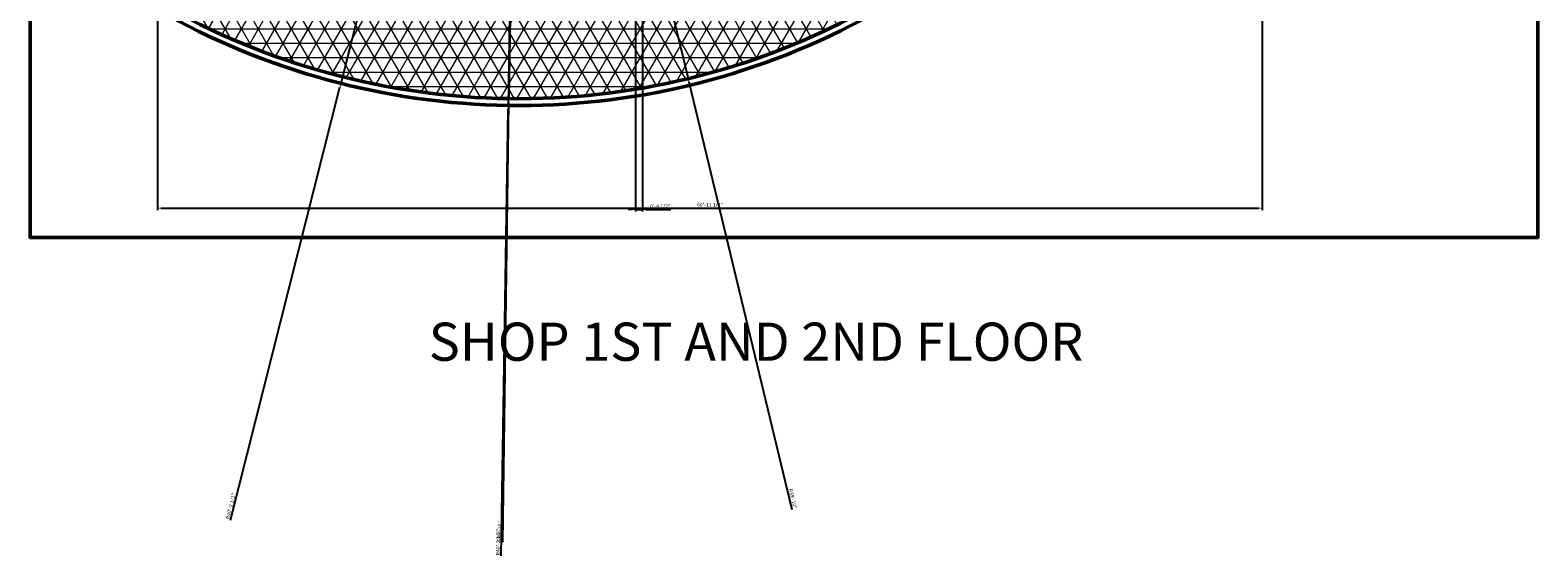
# Model space of a CAD drawing. Units: millimetres. Extents: x 1945 to 2943, y 628 to 2340.
# Tile 1 of 5: x 1945 to 2943, y 628 to 977. Entities that reach past the tile are written whole.
import ezdxf

# ---------------------------------------------------------------- set-up
doc = ezdxf.new("R2010")
doc.units = ezdxf.units.MM
for name, color, linetype, lineweight in [('A-ANNO-DIMS', 2, 'Continuous', 18), ('A-ANNO-TEXT', 7, 'Continuous', 18), ('A-FLOR-PATT', 8, 'Continuous', 13), ('A-WALL', 7, 'Continuous', 50)]:
    doc.layers.add(name, color=color, linetype=linetype, lineweight=lineweight)
doc.styles.get("Standard").update_dxf_attribs({"font": 'arial.ttf'})
doc.styles.add('YQ_IDEN', font='COMPLEX.SHX', dxfattribs={"bigfont": 'GBCBIG.SHX'})
doc.dimstyles.new('ISO-25', dxfattribs={"dimtxt": 2.5, "dimasz": 2.5, "dimexe": 1.25, "dimexo": 0.625, "dimtad": 1, "dimlunit": 3, "dimtxsty": 'Standard', "dimcen": 2.5, "dimadec": 0, "dimazin": 0, "dimtfac": 1, "dimtmove": 0, "dimatfit": 3, "dimfxl": 1, "dimarcsym": 0})

# ---------------------------------------------------------------- blocks, each defined once
blk = doc.blocks.new('*D24')
at = {"layer": 'A-ANNO-DIMS', "color": 0, "lineweight": -2, "transparency": 16777216}
for p, q in [((2760.6, 1123.5), (2760.6, 857.56)), ((2029.02, 989.8), (2029.02, 857.56)), ((2031.52, 858.81), (2758.1, 858.81))]:
    blk.add_line(p, q, dxfattribs=at)
at = {"layer": 'A-ANNO-DIMS', "color": 0, "transparency": 16777216}
for points in [[(2031.52, 859.23), (2031.52, 858.39), (2029.02, 858.81)], [(2758.1, 859.23), (2758.1, 858.39), (2760.6, 858.81)]]:
    blk.add_solid(points, dxfattribs=at)
at = {"layer": 'Defpoints', "color": 0, "transparency": 16777216}
for p in [(2760.6, 1124.12), (2029.02, 990.43), (2760.6, 858.81)]:
    blk.add_point(p, dxfattribs=at)
at = {"layer": 'A-ANNO-DIMS', "color": 0, "transparency": 16777216, "insert": (2394.81, 860.73), "char_height": 2.5, "attachment_point": 5}
blk.add_mtext('60\'-11 1/2"', dxfattribs=at)
blk = doc.blocks.new('*D25')
at = {"layer": 'A-ANNO-DIMS', "color": 0, "lineweight": -2, "transparency": 16777216}
for p, q in [((2268.43, 1409.46), (2261.15, 926.91)), ((2256.65, 628.35), (2261.11, 924.41))]:
    blk.add_line(p, q, dxfattribs=at)
at = {"layer": 'A-ANNO-DIMS', "color": 0, "transparency": 16777216}
blk.add_solid([(2260.7, 924.42), (2261.53, 924.4), (2261.15, 926.91)], dxfattribs=at)
at = {"layer": 'Defpoints', "color": 0, "transparency": 16777216}
for p in [(2268.43, 1409.46), (2261.15, 926.91)]:
    blk.add_point(p, dxfattribs=at)
at = {"layer": 'A-ANNO-DIMS', "color": 0, "transparency": 16777216, "insert": (2254.87, 637.41), "char_height": 2.5, "attachment_point": 5, "rotation": 89.13551}
blk.add_mtext('R40\'-2 1/2"', dxfattribs=at)
blk = doc.blocks.new('*D26')
at = {"layer": 'A-ANNO-DIMS', "color": 0, "lineweight": -2, "transparency": 16777216}
for p, q in [((2268.43, 1409.46), (2261.71, 931.4)), ((2257.57, 637.48), (2261.67, 928.9))]:
    blk.add_line(p, q, dxfattribs=at)
at = {"layer": 'A-ANNO-DIMS', "color": 0, "transparency": 16777216}
blk.add_solid([(2261.26, 928.91), (2262.09, 928.9), (2261.71, 931.4)], dxfattribs=at)
at = {"layer": 'Defpoints', "color": 0, "transparency": 16777216}
for p in [(2268.43, 1409.46), (2261.71, 931.4)]:
    blk.add_point(p, dxfattribs=at)
at = {"layer": 'A-ANNO-DIMS', "color": 0, "transparency": 16777216, "insert": (2255.77, 644.6), "char_height": 2.5, "attachment_point": 5, "rotation": 89.19401}
blk.add_mtext('R39\'-10"', dxfattribs=at)
blk = doc.blocks.new('*D30')
at = {"layer": 'A-ANNO-DIMS', "color": 0, "lineweight": -2, "transparency": 16777216}
for p, q in [((2345.6, 2086), (2345.6, 856.56)), ((2350.1, 2086), (2350.1, 856.56)), ((2343.1, 857.81), (2340.6, 857.81)), ((2345.6, 857.81), (2350.1, 857.81)), ((2352.6, 857.81), (2368.82, 857.81))]:
    blk.add_line(p, q, dxfattribs=at)
at = {"layer": 'A-ANNO-DIMS', "color": 0, "transparency": 16777216}
for points in [[(2343.1, 858.23), (2343.1, 857.39), (2345.6, 857.81)], [(2352.6, 858.23), (2352.6, 857.39), (2350.1, 857.81)]]:
    blk.add_solid(points, dxfattribs=at)
at = {"layer": 'Defpoints', "color": 0, "transparency": 16777216}
for p in [(2345.6, 2086.62), (2350.1, 2086.62), (2350.1, 857.81)]:
    blk.add_point(p, dxfattribs=at)
at = {"layer": 'A-ANNO-DIMS', "color": 0, "transparency": 16777216, "insert": (2361.96, 859.73), "char_height": 2.5, "attachment_point": 5}
blk.add_mtext('0\'-4 1/2"', dxfattribs=at)
blk = doc.blocks.new('*D31')
at = {"layer": 'A-ANNO-DIMS', "color": 0, "lineweight": -2, "transparency": 16777216}
for p, q in [((2268.43, 1409.46), (2150.43, 941.5)), ((2077.42, 651.98), (2149.82, 939.08))]:
    blk.add_line(p, q, dxfattribs=at)
at = {"layer": 'A-ANNO-DIMS', "color": 0, "transparency": 16777216}
blk.add_solid([(2149.41, 939.18), (2150.22, 938.98), (2150.43, 941.5)], dxfattribs=at)
at = {"layer": 'Defpoints', "color": 0, "transparency": 16777216}
for p in [(2268.43, 1409.46), (2150.43, 941.5)]:
    blk.add_point(p, dxfattribs=at)
at = {"layer": 'A-ANNO-DIMS', "color": 0, "transparency": 16777216, "insert": (2077.77, 661.2), "char_height": 2.5, "attachment_point": 5, "rotation": 75.84677}
blk.add_mtext('R40\'-2 1/2"', dxfattribs=at)
blk = doc.blocks.new('*D32')
at = {"layer": 'A-ANNO-DIMS', "color": 0, "lineweight": -2, "transparency": 16777216}
for p, q in [((2268.43, 1409.46), (2380.4, 944.65)), ((2449.24, 658.88), (2380.98, 942.22))]:
    blk.add_line(p, q, dxfattribs=at)
at = {"layer": 'A-ANNO-DIMS', "color": 0, "transparency": 16777216}
blk.add_solid([(2381.39, 942.32), (2380.58, 942.12), (2380.4, 944.65)], dxfattribs=at)
at = {"layer": 'Defpoints', "color": 0, "transparency": 16777216}
for p in [(2268.43, 1409.46), (2380.4, 944.65)]:
    blk.add_point(p, dxfattribs=at)
at = {"layer": 'A-ANNO-DIMS', "color": 0, "transparency": 16777216, "insert": (2449.43, 666.21), "char_height": 2.5, "attachment_point": 5, "rotation": 283.5436}
blk.add_mtext('R39\'-10"', dxfattribs=at)

msp = doc.modelspace()

# ---------------------------------------------------------------- hatches: boundary and pattern name
at = {"layer": 'A-FLOR-PATT'}
h = msp.add_hatch(dxfattribs=at)
h.set_pattern_fill('NET3', color=256, scale=3)
h.set_pattern_definition([(0, (1094.862, 577.549), (0, 9.525), []), (60, (1094.862, 577.549), (-8.24889, 4.7625), []), (120, (1094.862, 577.549), (-8.24889, -4.7625), [])])
h.paths.add_polyline_path([(2490.597, 1124.121), (2184.097, 1124.121), (2184.097, 1070.121), (2059.269, 1104.268), (2037.334, 990.918, 0.252088), (2490.597, 986.107)])

# ---------------------------------------------------------------- linework, layer by layer
at = {"layer": 'A-WALL', "ltscale": 0.5}
msp.add_lwpolyline([(1944.667, 2340.145), (2943.065, 2340.145), (2943.065, 839.363), (1944.667, 839.363)], close=True, dxfattribs=at)
at = {"layer": 'A-WALL'}
for radius, start, end in [(482.602, 240.258112, 298.012953), (478.102, 240.087713, 298.300235)]:
    msp.add_arc((2268.433, 1409.456), radius, start, end, dxfattribs=at)

# ---------------------------------------------------------------- texts
at = {"layer": 'A-ANNO-TEXT', "ltscale": 0.5, "insert": (2208.612, 782.957), "char_height": 25.33, "attachment_point": 1, "style": 'YQ_IDEN'}
msp.add_mtext_dynamic_manual_height_columns('SHOP 1ST AND 2ND FLOOR', width=658.32978, gutter_width=12.5, heights=[0], dxfattribs=at)

# ---------------------------------------------------------------- dimensions: what is measured, and where the dimension line sits
at = {"layer": 'A-ANNO-DIMS'}
for base, p1, p2, picture, middle in [((2350.097, 857.809), (2345.597, 2086.621), (2350.097, 2086.621), '*D30', (2361.958, 859.727)), ((2760.597, 858.809), (2029.018, 990.428), (2760.597, 1124.121), '*D24', (2394.808, 860.727))]:
    dim = msp.add_linear_dim(base=base, p1=p1, p2=p2, dimstyle='ISO-25', override={"dimdec": 1, "dimlfac": 1, "dimrnd": 0, "dimzin": 1, "dimdsep": 46, "dimlunit": 4, "dimfrac": 2}, dxfattribs=at)
    dim.commit()
    dim.dimension.update_dxf_attribs({"geometry": picture, "text_midpoint": middle})
for mpoint, picture, middle in [((2150.43, 941.503), '*D31', (2079.627, 660.732)), ((2261.152, 926.909), '*D25', (2256.783, 637.381)), ((2261.708, 931.402), '*D26', (2257.673, 644.569)), ((2380.398, 944.649), '*D32', (2447.576, 665.765))]:
    dim = msp.add_radius_dim(center=(2268.433, 1409.456), mpoint=mpoint, dimstyle='ISO-25', override={"dimdec": 1, "dimlfac": 1, "dimrnd": 0, "dimzin": 1, "dimdsep": 46, "dimlunit": 4, "dimfrac": 2}, dxfattribs=at)
    dim.commit()
    dim.dimension.update_dxf_attribs({"geometry": picture, "text_midpoint": middle, "dimtype": 164})

doc.saveas('drawing.dxf')
